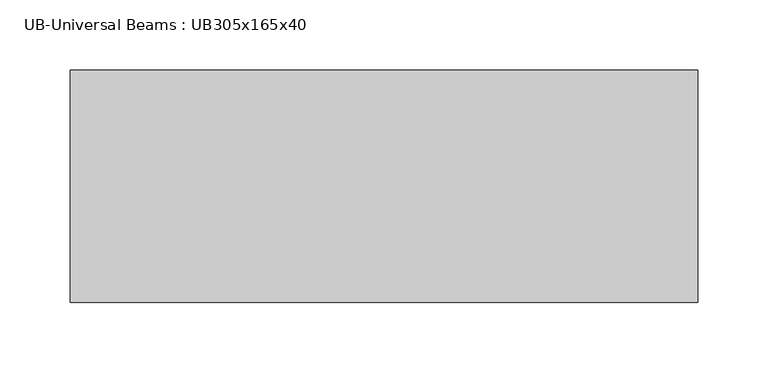
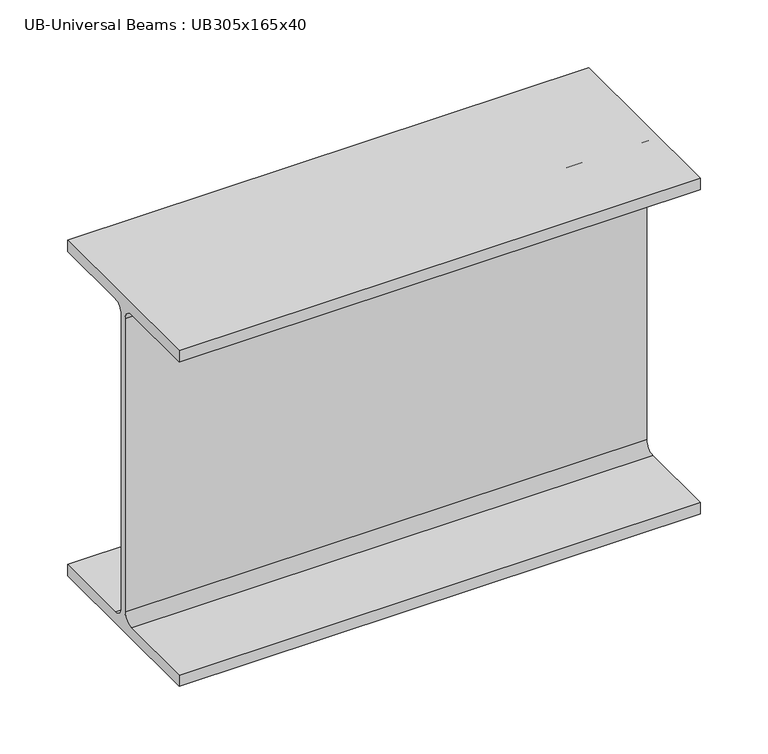
"""IFC4 building model written with IfcOpenShell, lengths in millimetres: beam geometry, UB-Universal Beams : UB305x165x40."""

from ifc_helpers import new_model, si_unit, point, frame, frame_2d, origin, place, context, project, spatial, polyline, circle_curve, trimmed, segment, composite_curve, outline, extrude, source, transform, mapped, element, save


def ub_universal_beams_ub305x165x40_07ff8ca2(model_context):
    return source(origin(), model_context, "Body", "SweptSolid", [
        extrude(outline(composite_curve([segment(polyline([(82.5, -141.5), (82.5, -151.7), (-82.5, -151.7), (-82.5, -141.5), (-11.9, -141.5)]), True, "CONTINUOUS"), segment(trimmed(circle_curve(frame_2d((-11.9, -132.6)), 8.9), [point((-11.9, -141.5))], [point((-3.0, -132.6))], True, "CARTESIAN"), True, "CONTINUOUS"), segment(polyline([(-3.0, -132.6), (-3.0, 132.6)]), True, "CONTINUOUS"), segment(trimmed(circle_curve(frame_2d((-11.9, 132.6)), 8.9), [point((-3.0, 132.6))], [point((-11.9, 141.5))], True, "CARTESIAN"), True, "CONTINUOUS"), segment(polyline([(-11.9, 141.5), (-82.5, 141.5), (-82.5, 151.7), (82.5, 151.7), (82.5, 141.5), (11.9, 141.5)]), True, "CONTINUOUS"), segment(trimmed(circle_curve(frame_2d((11.9, 132.6)), 8.9), [point((11.9, 141.5))], [point((3.0, 132.6))], True, "CARTESIAN"), True, "CONTINUOUS"), segment(polyline([(3.0, 132.6), (3.0, -132.6)]), True, "CONTINUOUS"), segment(trimmed(circle_curve(frame_2d((11.9, -132.6)), 8.9), [point((3.0, -132.6))], [point((11.9, -141.5))], True, "CARTESIAN"), True, "CONTINUOUS"), segment(polyline([(11.9, -141.5), (82.5, -141.5)]), True, "CONTINUOUS")], self_intersect=False)), frame((-235.6, 0.0, 0.0), z_axis=(1.0, 0.0, 0.0), x_axis=(0.0, 1.0, 0.0)), (0.0, 0.0, 1.0), 445.4),
    ])


if __name__ == "__main__":
    model = new_model("IFC4")
    model_context = context("Model", 3, world=origin())
    ifc_project = project(units=[si_unit("LENGTHUNIT", "METRE", prefix="MILLI")], contexts=[model_context])
    site = spatial("IfcSite", under=ifc_project)
    building = spatial("IfcBuilding", under=site)
    placement = place(None, origin())
    ub_universal_beams_ub305x165x40_shape = ub_universal_beams_ub305x165x40_07ff8ca2(model_context)
    element("IfcBeam", 1, ObjectType="UB-Universal Beams : UB305x165x40", at=placement, inside=building, context=model_context, shape_type="MappedRepresentation", body=[
        mapped(ub_universal_beams_ub305x165x40_shape, transform((0.0, 0.0, 0.0), x_axis=(1.0, 0.0, 0.0), y_axis=(0.0, 1.0, 0.0), z_axis=(0.0, 0.0, 1.0))),
    ])
    save(model, "model.ifc")

# Revit data of these elements
# Type "UB-Universal Beams : UB305x165x40"
#   Section Name Key = "UB305X165X40"
#   Width = 16.5 cm
#   Web Thickness = 0.6 cm
#   Web Fillet = 0.89 cm
#   Warping Constant = 164000.0 cm⁶
#   Torsional Moment of Inertia = 14.70 cm⁴
#   Section Area = 51.3 cm²
#   Plastic Modulus weak axis = 142.0 cm³
#   Plastic Modulus strong axis = 623.0 cm³
#   Nominal Weight = 40.2999 kgf/m
#   Moment of Inertia weak axis = 764.00 cm⁴
#   Moment of Inertia strong axis = 8503.00 cm⁴
#   Height = 30.34 cm
#   Flange Thickness = 1.02 cm
#   Elastic Modulus weak axis = 92.6 cm³
#   Elastic Modulus strong axis = 560.0 cm³
#   Centroid Vertical = 15.17 cm
#   Centroid Horizontal = 8.25 cm
#   Bolt Spacing = 9.0 cm
#   Length [instance default] = 1500 mm
#   Structural Material [instance default] = Metal - Steel 43-275
#   Type Comments = ""
#   Assembly Code = ""
# Element 1 (IfcBeam, "UB-Universal Beams : UB305x165x40")
#   Materials on its faces: "Metal - Steel 43-275"
# Materials
#   "Metal - Steel 43-275": class "Metal", colour RGB 247 247 247, transparency 0, Cost = 0
